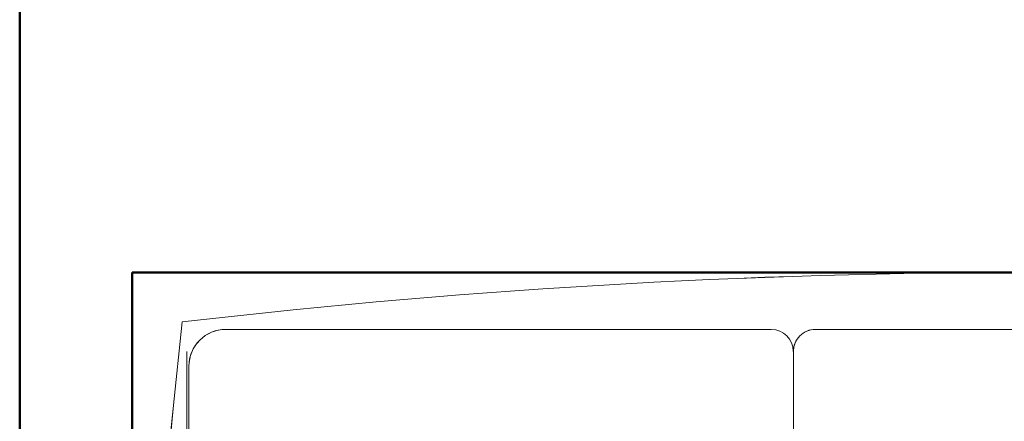
# Model space of a CAD drawing. Units: inches. Extents: x -466983 to 1020, y 324 to 318697.
# Tile 66 of 97: x 609 to 644, y 949 to 963. Entities that reach past the tile are written whole.
import ezdxf

# ---------------------------------------------------------------- set-up
doc = ezdxf.new("R2010")
doc.units = ezdxf.units.IN
doc.header["$MEASUREMENT"] = 0
for name, color, linetype, lineweight in [('A-FLOR-PATT', 252, 'Continuous', 13), ('A-FURN', 8, 'Continuous', 18), ('A-WALL', 7, 'Continuous', 50)]:
    doc.layers.add(name, color=color, linetype=linetype, lineweight=lineweight)

# ---------------------------------------------------------------- blocks, each defined once
blk = doc.blocks.new('L Shaped Sofa')
at = {"ltscale": 2}
for p, q in [((2475.263, 723.229), (2475.263, 821.686)), ((2471.575, 729.305), (2471.575, 765.138)), ((2432.347, 728.35), (2432.347, 736.259)), ((2471.701, 728.35), (2471.701, 736.259)), ((2430.914, 726.917), (2396.145, 726.917)), ((2469.187, 726.917), (2433.78, 726.917)), ((2475.263, 723.229), (2377.232, 723.229))]:
    blk.add_line(p, q, dxfattribs=at)
for centre, radius, start, end in [((1939.075, 785.436), 536.188, 353.68225, 6.54157), ((2469.187, 729.305), 2.388, 270, 0), ((2430.914, 728.35), 1.433, 270, 0), ((2433.78, 728.35), 1.433, 180, 270), ((2416.36, 1205.029), 481.82, 262.88673, 276.63201)]:
    blk.add_arc(centre, radius, start, end, dxfattribs=at)

msp = doc.modelspace()

# ---------------------------------------------------------------- hatches: boundary and pattern name
at = {"layer": 'A-FLOR-PATT', "transparency": 33554572}
h = msp.add_hatch(dxfattribs=at)
h.set_pattern_fill('ANSI37', color=256, scale=30)
h.set_pattern_definition([(45, (-1212.4137, -290.035), (-2.6516504, 2.6516504), []), (135, (-1212.4137, -290.035), (-2.6516504, -2.6516504), [])])
h.paths.add_polyline_path([(901.806, 1075.938), (900.614, 1075.938), (900.614, 1065.386), (899.391, 1065.386), (898.091, 1065.386), (892.836, 1058.71, -0.258377), (892.188, 1058.351), (879.985, 1058.351, -0.20177), (879.438, 1058.581), (874.081, 1065.386), (872.781, 1065.386), (871.558, 1065.386), (871.558, 1075.938), (813.806, 1075.938), (813.806, 1044.792), (832.395, 1044.792, -0.394795), (848.66, 1028.536), (848.66, 1009.938), (901.806, 1009.938), (901.806, 1015.938), (901.306, 1015.938), (871.306, 1015.938), (871.306, 1017.25), (871.334, 1017.25, -0.401453), (901.306, 1045.938), (901.806, 1045.938)])
edge = h.paths.add_edge_path(flags=16)
edge.add_line((847.773, 1068.949), (847.773, 1073.709))
edge.add_arc((849.227, 1073.709), 1.454, 90, 180, ccw=False)
edge.add_line((849.227, 1075.163), (864.492, 1075.163))
edge.add_arc((864.492, 1073.709), 1.454, 0, 90, ccw=False)
edge.add_line((865.946, 1073.709), (865.946, 1069.004))
edge.add_arc((832.645, 1068.976), 33.301, -20.6123, 0.0472, ccw=False)
edge.add_ellipse((856.859, 1058.48), major_axis=(0, 10.213), ratio=0.685919, start_angle=100.0088, end_angle=259.9912, ccw=False)
edge.add_arc((881.074, 1068.976), 33.301, 180.0472, 200.6123, ccw=False)
h.paths.add_polyline_path([(853.146, 1066.482), (853.146, 1066.453), (853.146, 1066.453, 0.433107), (852.917, 1066.685), (852.917, 1066.453), (853.146, 1066.453), (853.146, 1066.482), (853.088, 1066.612, 0.697939), (852.7, 1066.453), (852.7, 1066.453), (852.7, 1066.482), (852.917, 1067.001), (852.917, 1066.685, -0.396254)], flags=0)
h.paths.add_polyline_path([(861.019, 1066.482), (861.019, 1066.453), (861.019, 1066.453, 0.416404), (860.802, 1066.685), (860.802, 1066.453), (861.019, 1066.453), (861.019, 1066.482), (860.967, 1066.605, 0.713344), (860.573, 1066.453), (860.573, 1066.453), (860.573, 1066.482), (860.802, 1067.001), (860.802, 1066.685, -0.379973)], flags=0)
edge = h.paths.add_edge_path(flags=0)
edge.add_spline(control_points=[(861.13, 1065.785), (861.466, 1065.248), (861.613, 1065.016), (861.983, 1064.374), (862.192, 1063.944), (862.561, 1063.039), (862.721, 1062.563), (862.987, 1061.578), (863.092, 1061.069), (863.245, 1060.031), (863.293, 1059.503), (863.329, 1058.441), (863.318, 1057.908), (863.237, 1056.852), (863.166, 1056.329), (862.97, 1055.308), (862.843, 1054.81), (862.537, 1053.852), (862.357, 1053.393), (861.951, 1052.525), (861.725, 1052.117), (861.233, 1051.362), (860.967, 1051.016), (860.405, 1050.395), (860.108, 1050.12), (859.494, 1049.646), (859.176, 1049.448), (858.528, 1049.13), (858.197, 1049.011), (857.531, 1048.852), (857.196, 1048.812), (856.525, 1048.812), (856.189, 1048.852), (855.524, 1049.01), (855.193, 1049.129), (854.545, 1049.447), (854.227, 1049.645), (853.612, 1050.118), (853.316, 1050.393), (852.753, 1051.014), (852.487, 1051.36), (851.995, 1052.114), (851.769, 1052.523), (851.363, 1053.39), (851.183, 1053.85), (850.877, 1054.807), (850.75, 1055.305), (850.553, 1056.326), (850.483, 1056.849), (850.401, 1057.905), (850.39, 1058.438), (850.426, 1059.5), (850.473, 1060.028), (850.626, 1061.066), (850.732, 1061.575), (850.997, 1062.561), (851.157, 1063.036), (851.525, 1063.942), (851.734, 1064.371), (852.106, 1065.016), (852.254, 1065.25), (852.608, 1065.733)], knot_values=[3.915332, 3.915332, 3.915332, 3.915332, 4.013468, 4.013468, 4.175532, 4.175532, 4.337596, 4.337596, 4.49966, 4.49966, 4.661724, 4.661724, 4.823788, 4.823788, 4.985852, 4.985852, 5.147916, 5.147916, 5.30998, 5.30998, 5.472044, 5.472044, 5.634109, 5.634109, 5.796173, 5.796173, 5.958237, 5.958237, 6.120301, 6.120301, 6.282365, 6.282365, 6.444429, 6.444429, 6.606493, 6.606493, 6.768557, 6.768557, 6.930621, 6.930621, 7.092685, 7.092685, 7.254749, 7.254749, 7.416813, 7.416813, 7.578878, 7.578878, 7.740942, 7.740942, 7.903006, 7.903006, 8.06507, 8.06507, 8.227134, 8.227134, 8.389198, 8.389198, 8.551262, 8.551262, 8.65037, 8.65037, 8.65037, 8.65037], degree=3, periodic=0)
edge.add_line((852.642, 1065.785), (861.13, 1065.785))
edge = h.paths.add_edge_path(flags=0)
edge.add_ellipse((856.85, 1057.743), major_axis=(0, 7.792), ratio=0.687861, start_angle=0, end_angle=360)
h.paths.add_polyline_path([(848.863, 1069.389), (848.863, 1073.96, -0.414214), (849.954, 1075.051), (863.765, 1075.051, -0.414214), (864.856, 1073.96), (864.856, 1069.389, -0.388936), (864.524, 1069.027, -0.043561), (849.195, 1069.027, -0.388936)], flags=0)
h.paths.add_polyline_path([(853.101, 1068.112, -1), (852.677, 1068.112, -1)], flags=0)
edge = h.paths.add_edge_path(flags=0)
edge.add_ellipse((856.859, 1057.338), major_axis=(0, 2.207), ratio=0.657164, start_angle=0, end_angle=360)
h.paths.add_polyline_path([(861.041, 1068.112, -1), (860.618, 1068.112, -1)], flags=0)
edge = h.paths.add_edge_path()
edge.add_line((573.954, 1057.341), (573.954, 1075.938))
edge.add_line((573.954, 1075.938), (558.731, 1075.938))
edge.add_line((558.731, 1075.938), (558.731, 1065.386))
edge.add_line((558.731, 1065.386), (557.507, 1065.386))
edge.add_line((557.507, 1065.386), (556.207, 1065.386))
edge.add_line((556.207, 1065.386), (550.952, 1058.71))
edge.add_arc((550.304, 1059.116), 0.765, 270, 327.9483, ccw=False)
edge.add_line((550.304, 1058.351), (538.101, 1058.351))
edge.add_arc((538.101, 1059.116), 0.765, 224.3704, 270, ccw=False)
edge.add_line((537.555, 1058.581), (532.198, 1065.386))
edge.add_line((532.198, 1065.386), (530.898, 1065.386))
edge.add_line((530.898, 1065.386), (529.674, 1065.386))
edge.add_line((529.674, 1065.386), (529.674, 1075.938))
edge.add_line((529.674, 1075.938), (520.806, 1075.938))
edge.add_line((520.806, 1075.938), (520.806, 1045.938))
edge.add_line((520.806, 1045.938), (521.306, 1045.938))
edge.add_arc((521.306, 1015.938), 30, 2.5075, 90, ccw=False)
edge.add_line((551.277, 1017.25), (551.306, 1017.25))
edge.add_line((551.306, 1017.25), (551.306, 1015.938))
edge.add_line((551.306, 1015.938), (520.806, 1015.938))
edge.add_line((520.806, 1015.938), (520.806, 1009.938))
edge.add_line((520.806, 1009.938), (559.191, 1010.402))
edge.add_arc((559.191, 1011.856), 1.454, 180, 270, ccw=False)
edge.add_line((557.737, 1011.856), (557.737, 1016.561))
edge.add_arc((591.039, 1016.589), 33.301, 159.3877, 180.0472, ccw=False)
edge.add_ellipse((566.824, 1027.085), major_axis=(0, 10.213), ratio=0.685919, start_angle=280.0088, end_angle=439.9912, ccw=False)
edge.add_arc((542.609, 1016.589), 33.301, 0.0472, 20.6123, ccw=False)
edge.add_line((575.91, 1016.616), (575.91, 1011.856))
edge.add_arc((574.456, 1011.856), 1.454, -90, 0, ccw=False)
edge.add_line((574.456, 1010.402), (608.806, 1009.938))
edge.add_line((608.806, 1009.938), (608.806, 1041.086))
edge.add_line((608.806, 1041.086), (590.218, 1041.086))
edge.add_arc((590.775, 1057.907), 16.831, 181.9277, 268.1032, ccw=False)
edge = h.paths.add_edge_path()
edge.add_ellipse((494.244, 583.62), major_axis=(0, 10.213), ratio=0.685919, start_angle=280.0088, end_angle=439.9912, ccw=False)
edge.add_arc((470.03, 573.124), 33.301, 0.0472, 20.6123, ccw=False)
edge.add_line((503.331, 573.152), (503.331, 568.392))
edge.add_arc((501.877, 568.392), 1.454, -90, 0, ccw=False)
edge.add_line((501.877, 566.938), (539.806, 566.938))
edge.add_line((539.806, 566.938), (539.806, 572.938))
edge.add_line((539.806, 572.938), (539.306, 572.938))
edge.add_line((539.306, 572.938), (509.306, 572.938))
edge.add_line((509.306, 572.938), (509.306, 574.25))
edge.add_line((509.306, 574.25), (509.334, 574.25))
edge.add_arc((539.306, 572.938), 30, 90, 177.4925, ccw=False)
edge.add_line((539.306, 602.938), (539.806, 602.938))
edge.add_line((539.806, 602.938), (539.806, 626.938))
edge.add_line((539.806, 626.938), (531.772, 626.938))
edge.add_line((531.772, 626.938), (531.772, 616.386))
edge.add_line((531.772, 616.386), (530.548, 616.386))
edge.add_line((530.548, 616.386), (529.249, 616.386))
edge.add_line((529.249, 616.386), (523.711, 609.351))
edge.add_line((523.711, 609.351), (510.777, 609.351))
edge.add_line((510.777, 609.351), (505.239, 616.386))
edge.add_line((505.239, 616.386), (503.939, 616.386))
edge.add_line((503.939, 616.386), (502.715, 616.386))
edge.add_line((502.715, 616.386), (502.715, 626.938))
edge.add_line((502.715, 626.938), (481.698, 626.938))
edge.add_line((481.698, 626.938), (481.698, 610.995))
edge.add_arc((467.27, 611.473), 14.436, 271.9277, 358.1032, ccw=False)
edge.add_line((467.756, 597.045), (451.806, 597.045))
edge.add_line((451.806, 597.045), (451.806, 584.404))
edge.add_line((451.806, 584.404), (451.806, 566.938))
edge.add_line((451.806, 566.938), (486.612, 566.938))
edge.add_arc((486.612, 568.392), 1.454, 180, 270, ccw=False)
edge.add_line((485.158, 568.392), (485.158, 573.097))
edge.add_arc((518.459, 573.124), 33.301, 159.3877, 180.0472, ccw=False)
h.paths.add_polyline_path([(836.261, 1020.733), (879.89, 1020.733), (879.89, 1039.39), (836.261, 1039.39)], flags=25)
h.paths.add_polyline_path([(549.985, 1036.749), (593.614, 1036.749), (593.614, 1055.407), (549.985, 1055.407)], flags=24)
h.paths.add_polyline_path([(475.123, 595.596), (518.752, 595.596), (518.752, 614.253), (475.123, 614.253)], flags=24)
h = msp.add_hatch(dxfattribs=at)
h.set_pattern_fill('ANSI37', color=256, scale=20)
h.set_pattern_definition([(45, (-1212.4137, -290.035), (-1.767767, 1.767767), []), (135, (-1212.4137, -290.035), (-1.767767, -1.767767), [])])
h.paths.add_polyline_path([(809.806, 870.938), (809.806, 888.152), (806.998, 888.152), (802.662, 888.152), (789.383, 888.152), (786.285, 888.152, -0.414214), (785.499, 888.937), (785.499, 900.196), (785.499, 908.47, -0.414214), (786.808, 909.779, -0.414214), (785.499, 911.088), (785.499, 929.101, -0.414214), (786.808, 930.411, -0.414214), (785.499, 931.72), (785.499, 931.904, -0.414214), (784.19, 930.595), (766.722, 930.595, -0.412359), (765.413, 931.896, -0.413741), (764.115, 930.578), (744.578, 930.422, -0.416556), (743.786, 931.207), (743.786, 933.515), (742.215, 933.515), (742.215, 952.024, -0.001344), (743.786, 952.2), (743.786, 953.938), (678.592, 953.938), (678.592, 951.131), (678.592, 946.794), (678.592, 933.515), (678.592, 930.417, -0.414214), (677.806, 929.631), (666.548, 929.631), (658.274, 929.631, -0.414214), (656.965, 930.94, -0.414214), (655.656, 929.631), (637.642, 929.631, -0.414214), (636.333, 930.94, -0.414214), (635.024, 929.631), (634.839, 929.631, -0.414214), (636.149, 928.322), (636.149, 910.854, -0.412359), (634.848, 909.545, -0.413741), (636.165, 908.247), (636.321, 888.71, -0.416556), (635.536, 887.918), (633.228, 887.918), (633.228, 886.347), (614.719, 886.347, -0.001344), (614.544, 887.918), (612.806, 887.918), (612.806, 834.938), (612.806, 752.938), (612.806, 748.938), (612.806, 697.938), (654.806, 697.938), (654.806, 701.938), (715.806, 701.938), (715.806, 737.435), (774.292, 737.435), (774.292, 795.938), (809.806, 795.938)])
h.paths.add_polyline_path([(679.276, 849.576, 0.102523), (682.148, 849.261, -0.080461), (694.543, 849.773, -0.283899), (694.482, 849.008, 0.136605), (694.407, 848.81, -0.030441), (694.543, 846.893), (694.543, 842.62), (694.543, 838.347, -0.028219), (694.425, 836.568), (694.425, 836.568, 0.196187), (694.446, 836.271, -0.302897), (694.543, 835.467, -0.080461), (682.148, 835.979, 0.102523), (679.276, 835.664, -0.58611), (678.646, 836.017), (678.646, 849.223, -0.58611)], flags=16)
h.paths.add_polyline_path([(679.517, 848.651, 0.699597), (679.476, 848.634, 1.20716), (679.194, 848.742, 0.010621)], flags=0)
h.paths.add_polyline_path([(679.492, 836.561, -0.013798), (679.918, 836.659, -0.071703), (682.853, 837.143, -0.165743), (682.166, 839.101), (682.166, 842.609), (682.166, 846.06, -0.240616), (683.473, 848.677, -0.068263), (693.929, 849.008), (693.788, 848.708), (693.788, 849.023, 0.067332), (683.473, 848.677, 0.240616), (682.166, 846.06), (682.166, 842.609), (682.166, 839.101, 0.23459), (683.461, 836.551, 0.068093), (693.788, 836.195), (693.788, 836.51), (693.93, 836.21, -0.077215), (682.242, 836.782, 0.086627), (679.528, 836.57, -0.628402), (679.503, 836.573), (679.503, 836.607, 0.910458)], flags=0)
h.paths.add_polyline_path([(679.476, 848.636), (679.207, 848.647), (679.207, 836.572, 0.913566), (679.365, 836.586), (679.476, 836.582)], flags=0)
h.paths.add_polyline_path([(679.276, 829.86, 0.102523), (682.148, 829.546, -0.080461), (694.543, 830.057, -0.283899), (694.482, 829.293, 0.136605), (694.407, 829.095, -0.030441), (694.543, 827.178), (694.543, 822.904), (694.543, 818.631, -0.028219), (694.425, 816.853), (694.425, 816.853, 0.196187), (694.446, 816.556, -0.302897), (694.543, 815.752, -0.080461), (682.148, 816.263, 0.102523), (679.276, 815.949, -0.58611), (678.646, 816.302), (678.646, 829.507, -0.58611)], flags=16)
h.paths.add_polyline_path([(679.517, 828.936, 0.699597), (679.476, 828.919, 1.20716), (679.194, 829.027, 0.010621)], flags=0)
h.paths.add_polyline_path([(679.492, 816.846, -0.013798), (679.918, 816.944, -0.071703), (682.853, 817.428, -0.165743), (682.166, 819.385), (682.166, 822.894), (682.166, 826.345, -0.240616), (683.473, 828.961, -0.068263), (693.929, 829.293), (693.788, 828.993), (693.788, 829.308, 0.067332), (683.473, 828.961, 0.240616), (682.166, 826.345), (682.166, 822.894), (682.166, 819.385, 0.23459), (683.461, 816.836, 0.068093), (693.788, 816.48), (693.788, 816.795), (693.93, 816.495, -0.077215), (682.242, 817.066, 0.086627), (679.528, 816.855, -0.628402), (679.503, 816.858), (679.503, 816.892, 0.910458)], flags=0)
h.paths.add_polyline_path([(679.476, 828.921), (679.207, 828.932), (679.207, 816.857, 0.913566), (679.365, 816.871), (679.476, 816.867)], flags=0)
h.paths.add_polyline_path([(679.276, 810.145, 0.102523), (682.148, 809.83, -0.080461), (694.543, 810.342, -0.3023), (694.447, 809.539, 0.10023), (694.406, 809.388, -0.03057), (694.543, 807.462), (694.543, 803.189), (694.543, 798.916, -0.03057), (694.406, 796.991, 0.10023), (694.447, 796.839, -0.3023), (694.543, 796.036, -0.080461), (682.148, 796.548, 0.102523), (679.276, 796.233, -0.58611), (678.646, 796.586), (678.646, 809.792, -0.58611)], flags=16)
h.paths.add_polyline_path([(679.517, 809.242, 0.699597), (679.476, 809.224, 1.20716), (679.194, 809.332, 0.010621)], flags=0)
h.paths.add_polyline_path([(679.492, 797.151, -0.013798), (679.918, 797.25, -0.071703), (682.853, 797.734, -0.165743), (682.166, 799.691), (682.166, 803.2), (682.166, 806.65, -0.239349), (683.461, 809.258, -0.072465), (694.447, 809.541, 0.197932), (694.425, 809.241), (693.788, 809.299), (693.788, 809.614, 0.068093), (683.461, 809.258, 0.239349), (682.166, 806.65), (682.166, 803.2), (682.166, 799.691, 0.235854), (683.473, 797.132, 0.067332), (693.788, 796.786), (693.788, 797.101), (694.425, 797.159, 0.197932), (694.447, 796.859, -0.080419), (682.156, 797.379, 0.083867), (679.528, 797.16, -0.628402), (679.503, 797.164), (679.503, 797.197, 0.910458)], flags=0)
h.paths.add_polyline_path([(679.207, 809.237), (679.207, 797.162, 0.913566), (679.365, 797.176), (679.476, 797.173), (679.476, 809.227)], flags=0)
h.paths.add_polyline_path([(695.364, 853.299), (728.223, 853.299), (728.223, 771.152), (695.364, 771.152)], flags=16)
h.paths.add_polyline_path([(696.021, 852.642), (727.566, 852.642), (727.566, 771.809), (696.021, 771.809)], flags=0)
h.paths.add_polyline_path([(679.276, 788.787, 0.102523), (682.148, 788.472, -0.080461), (694.543, 788.984, -0.3023), (694.447, 788.181, 0.10023), (694.406, 788.03, -0.03057), (694.543, 786.104), (694.543, 781.831), (694.543, 777.558, -0.03057), (694.406, 775.632, 0.10023), (694.447, 775.481, -0.3023), (694.543, 774.678, -0.080461), (682.148, 775.19, 0.102523), (679.276, 774.875, -0.58611), (678.646, 775.228), (678.646, 788.434, -0.58611)], flags=16)
h.paths.add_polyline_path([(679.517, 787.883, 0.699597), (679.476, 787.866, 1.20716), (679.194, 787.974, 0.010621)], flags=0)
h.paths.add_polyline_path([(679.492, 775.793, -0.013798), (679.918, 775.891, -0.071703), (682.853, 776.375, -0.165743), (682.166, 778.333), (682.166, 781.841), (682.166, 785.292, -0.239349), (683.461, 787.899, -0.072465), (694.447, 788.182, 0.197932), (694.425, 787.882), (693.788, 787.94), (693.788, 788.255, 0.068093), (683.461, 787.899, 0.239349), (682.166, 785.292), (682.166, 781.841), (682.166, 778.333, 0.235854), (683.473, 775.774, 0.067332), (693.788, 775.428), (693.788, 775.742), (694.425, 775.8, 0.197932), (694.447, 775.5, -0.080419), (682.156, 776.021, 0.083867), (679.528, 775.802, -0.628402), (679.503, 775.805), (679.503, 775.839, 0.910458)], flags=0)
h.paths.add_polyline_path([(679.207, 787.879), (679.207, 775.804, 0.913566), (679.365, 775.818), (679.476, 775.814), (679.476, 787.868)], flags=0)
h.paths.add_polyline_path([(704.641, 854.12, -0.080461), (705.153, 866.516, 0.102523), (704.838, 869.387, -0.58611), (705.191, 870.017), (718.397, 870.017, -0.58611), (718.75, 869.387, 0.102523), (718.435, 866.516, -0.080461), (718.946, 854.12, -0.3023), (718.144, 854.217, 0.10023), (717.992, 854.257, -0.03057), (716.067, 854.12), (711.794, 854.12), (707.521, 854.12, -0.03057), (705.595, 854.257, 0.10023), (705.444, 854.217, -0.3023)], flags=16)
h.paths.add_polyline_path([(717.846, 869.146, 0.699597), (717.829, 869.187, 1.20716), (717.937, 869.47, 0.010621)], flags=0)
h.paths.add_polyline_path([(705.463, 854.216, -0.080419), (705.984, 866.507, 0.083867), (705.765, 869.135, -0.628402), (705.768, 869.16), (705.802, 869.16, 0.910458), (705.756, 869.171, -0.013798), (705.854, 868.745, -0.071703), (706.338, 865.81, -0.165743), (708.295, 866.497), (711.804, 866.497), (715.255, 866.497, -0.239349), (717.862, 865.202, -0.072465), (718.145, 854.216, 0.197932), (717.845, 854.238), (717.903, 854.876), (718.218, 854.876, 0.068093), (717.862, 865.202, 0.239349), (715.255, 866.497), (711.804, 866.497), (708.295, 866.497, 0.235854), (705.737, 865.19, 0.067332), (705.391, 854.876), (705.705, 854.876), (705.763, 854.238, 0.197932)], flags=16)
h.paths.add_polyline_path([(705.766, 869.456, 0.913566), (705.781, 869.299), (705.777, 869.187), (717.831, 869.187), (717.842, 869.456)], flags=0)
h.paths.add_polyline_path([(729.045, 842.62), (729.045, 846.893, -0.03057), (729.182, 848.818, 0.10023), (729.141, 848.97, -0.3023), (729.045, 849.773, -0.080461), (741.44, 849.261, 0.102523), (744.311, 849.576, -0.58611), (744.942, 849.223), (744.942, 836.017, -0.58611), (744.311, 835.664, 0.102523), (741.44, 835.979, -0.080461), (729.045, 835.467, -0.3023), (729.141, 836.27, 0.10023), (729.182, 836.421, -0.03057), (729.045, 838.347)], flags=16)
h.paths.add_polyline_path([(744.111, 836.585, 1.20716), (744.394, 836.477, 0.010621), (744.07, 836.567, 0.699597)], flags=0)
h.paths.add_polyline_path([(729.141, 836.268, 0.197932), (729.162, 836.568), (729.8, 836.51), (729.8, 836.195, 0.068093), (740.126, 836.551, 0.239349), (741.421, 839.159), (741.421, 842.609), (741.421, 846.118, 0.235854), (740.114, 848.677, 0.067332), (729.8, 849.023), (729.8, 848.708), (729.162, 848.65, 0.197932), (729.141, 848.95, -0.080419), (741.432, 848.43, 0.083867), (744.059, 848.649, -0.628402), (744.085, 848.645), (744.085, 848.612, 0.910458), (744.095, 848.658, -0.013798), (743.67, 848.559, -0.071703), (740.734, 848.075, -0.165743), (741.421, 846.118), (741.421, 842.609), (741.421, 839.159, -0.239349), (740.126, 836.551, -0.072465)], flags=0)
h.paths.add_polyline_path([(729.045, 830.057, -0.080461), (741.44, 829.546, 0.102523), (744.311, 829.86, -0.58611), (744.942, 829.507), (744.942, 816.302, -0.58611), (744.311, 815.949, 0.102523), (741.44, 816.263, -0.080461), (729.045, 815.752, -0.3023), (729.141, 816.554, 0.10023), (729.182, 816.706, -0.03057), (729.045, 818.631), (729.045, 822.904), (729.045, 827.178, -0.03057), (729.182, 829.103, 0.10023), (729.141, 829.255, -0.3023)], flags=16)
h.paths.add_polyline_path([(744.111, 816.869, 1.20716), (744.394, 816.761, 0.010621), (744.07, 816.852, 0.699597)], flags=0)
h.paths.add_polyline_path([(729.141, 829.235, -0.080419), (741.432, 828.714, 0.083867), (744.059, 828.933, -0.628402), (744.085, 828.93), (744.085, 828.896, 0.910458), (744.095, 828.943, -0.013798), (743.67, 828.844, -0.071703), (740.734, 828.36, -0.165743), (741.421, 826.403), (741.421, 822.894), (741.421, 819.443, -0.239349), (740.126, 816.836, -0.072465), (729.141, 816.553, 0.197932), (729.162, 816.853), (729.8, 816.795), (729.8, 816.48, 0.068093), (740.126, 816.836, 0.239349), (741.421, 819.443), (741.421, 822.894), (741.421, 826.403, 0.235854), (740.114, 828.961, 0.067332), (729.8, 829.308), (729.8, 828.993), (729.162, 828.935, 0.197932)], flags=16)
h.paths.add_polyline_path([(729.045, 810.342, -0.080461), (741.44, 809.83, 0.102523), (744.311, 810.145, -0.58611), (744.942, 809.792), (744.942, 796.586, -0.58611), (744.311, 796.233, 0.102523), (741.44, 796.548, -0.080461), (729.045, 796.036, -0.283899), (729.105, 796.801, 0.136605), (729.181, 796.999, -0.030441), (729.045, 798.916), (729.045, 803.189), (729.045, 807.462, -0.028219), (729.163, 809.241), (729.162, 809.241, 0.196187), (729.142, 809.538, -0.302897)], flags=16)
h.paths.add_polyline_path([(744.111, 797.175, 1.20716), (744.394, 797.067, 0.010621), (744.07, 797.158, 0.699597)], flags=0)
h.paths.add_polyline_path([(741.345, 809.027, 0.086627), (744.059, 809.239, -0.628402), (744.085, 809.235), (744.085, 809.202, 0.910458), (744.095, 809.248, -0.013798), (743.67, 809.15, -0.071703), (740.734, 808.666, -0.165743), (741.421, 806.708), (741.421, 803.2), (741.421, 799.749, -0.240616), (740.114, 797.132, -0.068263), (729.658, 796.801), (729.8, 797.101), (729.8, 796.786, 0.067332), (740.114, 797.132, 0.240616), (741.421, 799.749), (741.421, 803.2), (741.421, 806.708, 0.23459), (740.126, 809.258, 0.068093), (729.8, 809.614), (729.8, 809.299), (729.658, 809.599, -0.077215)], flags=0)
h.paths.add_polyline_path([(704.641, 770.33, -0.283899), (705.405, 770.27, 0.136605), (705.603, 770.194, -0.030441), (707.521, 770.33), (711.794, 770.33), (716.067, 770.33, -0.028219), (717.845, 770.212), (717.845, 770.213, 0.196187), (718.143, 770.233, -0.302897), (718.946, 770.33, -0.080461), (718.435, 757.935, 0.102523), (718.75, 755.064, -0.58611), (718.397, 754.433), (705.191, 754.433, -0.58611), (704.838, 755.064, 0.102523), (705.153, 757.935, -0.080461)], flags=16)
h.paths.add_polyline_path([(705.762, 755.305, 0.699597), (705.779, 755.264, 1.20716), (705.671, 754.981, 0.010621)], flags=0)
h.paths.add_polyline_path([(705.405, 769.717), (705.705, 769.575), (705.391, 769.575, 0.067332), (705.737, 759.261, 0.240616), (708.353, 757.954), (711.804, 757.954), (715.313, 757.954, 0.23459), (717.862, 759.249, 0.068093), (718.218, 769.575), (717.903, 769.575), (718.203, 769.717, -0.077215), (717.632, 758.03, 0.086627), (717.843, 755.316, -0.628402), (717.84, 755.29), (717.806, 755.29, 0.910458), (717.853, 755.28, -0.013798), (717.754, 755.705, -0.071703), (717.27, 758.641, -0.165743), (715.313, 757.954), (711.804, 757.954), (708.353, 757.954, -0.240616), (705.737, 759.261, -0.068263)], flags=0)
h.paths.add_polyline_path([(729.045, 788.984, -0.080461), (741.44, 788.472, 0.102523), (744.311, 788.787, -0.58611), (744.942, 788.434), (744.942, 775.228, -0.58611), (744.311, 774.875, 0.102523), (741.44, 775.19, -0.080461), (729.045, 774.678, -0.283899), (729.105, 775.443, 0.136605), (729.181, 775.64, -0.030441), (729.045, 777.558), (729.045, 781.831), (729.045, 786.104, -0.028219), (729.163, 787.882), (729.162, 787.882, 0.196187), (729.142, 788.18, -0.302897)], flags=16)
h.paths.add_polyline_path([(744.111, 775.817, 1.20716), (744.394, 775.709, 0.010621), (744.07, 775.799, 0.699597)], flags=0)
h.paths.add_polyline_path([(741.345, 787.669, 0.086627), (744.059, 787.881, -0.628402), (744.085, 787.877), (744.085, 787.844, 0.910458), (744.095, 787.89, -0.013798), (743.67, 787.791, -0.071703), (740.734, 787.307, -0.165743), (741.421, 785.35), (741.421, 781.841), (741.421, 778.39, -0.240616), (740.114, 775.774, -0.068263), (729.658, 775.443), (729.8, 775.742), (729.8, 775.428, 0.067332), (740.114, 775.774, 0.240616), (741.421, 778.39), (741.421, 781.841), (741.421, 785.35, 0.23459), (740.126, 787.899, 0.068093), (729.8, 788.255), (729.8, 787.94), (729.658, 788.241, -0.077215)], flags=0)
h.paths.add_polyline_path([(744.111, 848.636), (744.111, 836.582), (744.381, 836.572), (744.381, 848.647, 0.913566), (744.223, 848.633)], flags=0)
h.paths.add_polyline_path([(744.223, 828.917), (744.111, 828.921), (744.111, 816.867), (744.381, 816.857), (744.381, 828.932, 0.913566)], flags=0)
h.paths.add_polyline_path([(717.831, 755.264), (705.777, 755.264), (705.766, 754.994), (717.842, 754.994, 0.913566), (717.827, 755.152)], flags=0)
h.paths.add_polyline_path([(744.223, 809.223), (744.111, 809.227), (744.111, 797.173), (744.381, 797.162), (744.381, 809.237, 0.913566)], flags=0)
h.paths.add_polyline_path([(744.111, 787.868), (744.111, 775.814), (744.381, 775.804), (744.381, 787.879, 0.913566), (744.223, 787.865)], flags=0)
h.paths.add_polyline_path([(678.877, 877.123), (737.613, 877.123), (737.613, 899.512), (678.877, 899.512)], flags=24)

# ---------------------------------------------------------------- linework, layer by layer
at = {"layer": 'A-FURN', "ltscale": 2}
for p, q in [((612.806, 953.938), (612.806, 899.962)), ((612.806, 953.938), (666.548, 953.938)), ((612.806, 953.938), (612.806, 899.962)), ((612.806, 953.938), (666.548, 953.938)), ((612.806, 953.938), (612.806, 899.962)), ((612.806, 953.938), (666.548, 953.938)), ((612.806, 953.938), (612.806, 899.962)), ((612.806, 953.938), (666.548, 953.938)), ((612.806, 953.938), (612.806, 899.962)), ((612.806, 953.938), (666.548, 953.938)), ((612.806, 953.938), (612.806, 899.962)), ((612.806, 953.938), (666.548, 953.938)), ((616.137, 951.916), (635.547, 951.916)), ((616.137, 951.916), (635.547, 951.916)), ((616.137, 951.916), (635.547, 951.916)), ((616.137, 951.916), (635.547, 951.916)), ((616.137, 951.916), (635.547, 951.916)), ((616.137, 951.916), (635.547, 951.916)), ((637.118, 951.916), (656.179, 951.916)), ((637.118, 951.916), (656.179, 951.916)), ((637.118, 951.916), (656.179, 951.916)), ((637.118, 951.916), (656.179, 951.916)), ((637.118, 951.916), (656.179, 951.916)), ((637.118, 951.916), (656.179, 951.916)), ((614.758, 951.131), (614.758, 946.794)), ((614.758, 951.131), (614.758, 946.794)), ((614.758, 951.131), (614.758, 946.794)), ((614.758, 951.131), (614.758, 946.794)), ((614.758, 951.131), (614.758, 946.794)), ((614.758, 951.131), (614.758, 946.794)), ((636.333, 951.131), (636.333, 946.794)), ((636.333, 951.131), (636.333, 946.794)), ((636.333, 951.131), (636.333, 946.794)), ((636.333, 951.131), (636.333, 946.794)), ((636.333, 951.131), (636.333, 946.794)), ((636.333, 951.131), (636.333, 946.794)), ((614.827, 950.607), (614.827, 930.963)), ((614.827, 950.607), (614.827, 930.963)), ((614.827, 950.607), (614.827, 930.963)), ((614.827, 950.607), (614.827, 930.963)), ((614.827, 950.607), (614.827, 930.963)), ((614.827, 950.607), (614.827, 930.963))]:
    msp.add_line(p, q, dxfattribs=at)
for centre, radius, start, end in [((645.097, 689.808), 264.141, 82.88673, 96.63201), ((645.097, 689.808), 264.141, 82.88673, 96.63201), ((645.097, 689.808), 264.141, 82.88673, 96.63201), ((645.097, 689.808), 264.141, 82.88673, 96.63201), ((645.097, 689.808), 264.141, 82.88673, 96.63201), ((645.097, 689.808), 264.141, 82.88673, 96.63201), ((906.752, 919.835), 293.946, 173.68225, 186.54157), ((906.752, 919.835), 293.946, 173.68225, 186.54157), ((906.752, 919.835), 293.946, 173.68225, 186.54157), ((906.752, 919.835), 293.946, 173.68225, 186.54157), ((906.752, 919.835), 293.946, 173.68225, 186.54157), ((906.752, 919.835), 293.946, 173.68225, 186.54157), ((616.137, 950.607), 1.309, 90, 180), ((616.137, 950.607), 1.309, 90, 180), ((616.137, 950.607), 1.309, 90, 180), ((616.137, 950.607), 1.309, 90, 180), ((616.137, 950.607), 1.309, 90, 180), ((616.137, 950.607), 1.309, 90, 180), ((635.547, 951.131), 0.785, 0, 90), ((635.547, 951.131), 0.785, 0, 90), ((635.547, 951.131), 0.785, 0, 90), ((635.547, 951.131), 0.785, 0, 90), ((635.547, 951.131), 0.785, 0, 90), ((635.547, 951.131), 0.785, 0, 90), ((637.118, 951.131), 0.785, 90, 180), ((637.118, 951.131), 0.785, 90, 180), ((637.118, 951.131), 0.785, 90, 180), ((637.118, 951.131), 0.785, 90, 180), ((637.118, 951.131), 0.785, 90, 180), ((637.118, 951.131), 0.785, 90, 180)]:
    msp.add_arc(centre, radius, start, end, dxfattribs=at)
at = {"layer": 'A-WALL'}
for p, q in [((608.806, 870.938), (608.806, 1005.938)), ((612.806, 953.938), (680.592, 953.938)), ((612.806, 870.938), (612.806, 953.938))]:
    msp.add_line(p, q, dxfattribs=at)

# ---------------------------------------------------------------- block references
at = {"layer": 'A-FURN', "xscale": 0.5482153745360612, "yscale": 0.5482153745360612, "zscale": 0.5482153745360612, "rotation": 180}
msp.add_blockref('L Shaped Sofa', (1969.783, 1350.423), dxfattribs=at)

doc.saveas('drawing.dxf')
